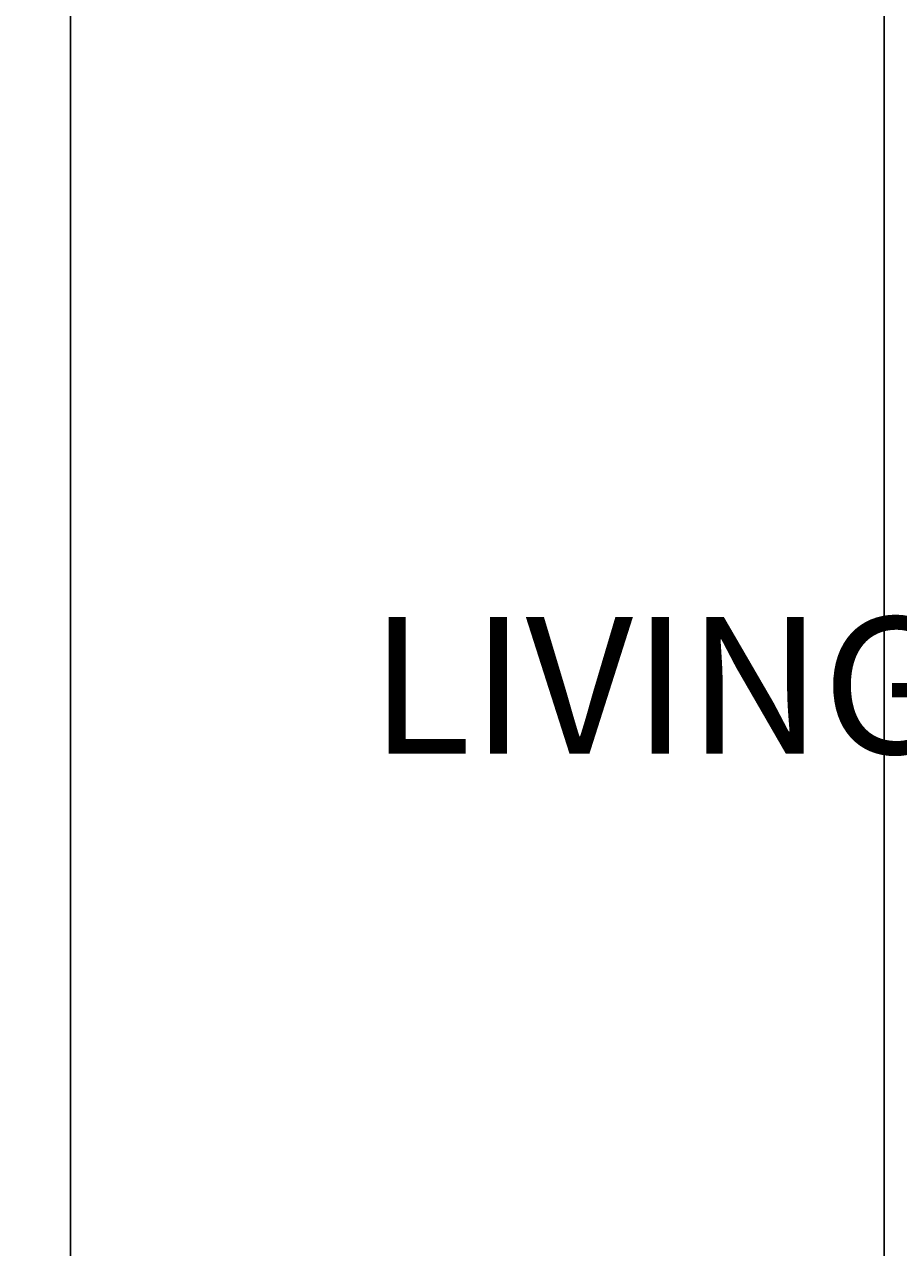
# Model space of a CAD drawing. Units: inches. Extents: x 857 to 1111, y 424 to 822.
# Tile 4 of 9: x 983 to 1031, y 600 to 668. Entities that reach past the tile are written whole.
import ezdxf

# ---------------------------------------------------------------- set-up
doc = ezdxf.new("R2010")
doc.units = ezdxf.units.IN
doc.layers.add('A-ANNO-DIMS', color=2, linetype='Continuous', lineweight=18)
doc.layers.add('A-AREA-IDEN', color=7, linetype='Continuous', lineweight=25)
doc.styles.get("Standard").update_dxf_attribs({"font": 'arial.ttf'})
doc.dimstyles.get("Standard").update_dxf_attribs({"dimtxt": 0.18, "dimasz": 0.18, "dimexe": 0.18, "dimexo": 0.0625, "dimgap": 0.09, "dimtad": 0, "dimtih": 1, "dimtoh": 1, "dimdec": 4, "dimzin": 0, "dimdsep": 46, "dimtxsty": 'Standard', "dimcen": 0.09, "dimadec": 0, "dimazin": 0, "dimtfac": 1, "dimtdec": 4, "dimtofl": 0, "dimtmove": 0, "dimatfit": 3, "dimfxl": 1, "dimtolj": 1, "dimtzin": 0, "dimarcsym": 0})

# ---------------------------------------------------------------- blocks, each defined once
blk = doc.blocks.new('*D48')
at = {"layer": 'A-ANNO-DIMS', "color": 0, "lineweight": -2, "transparency": 16777216}
for p, q in [((885.137, 582.419), (885.137, 822.087)), ((885.317, 821.907), (935.001, 821.907)), ((985.457, 821.907), (935.773, 821.907)), ((985.637, 582.419), (985.637, 822.087))]:
    blk.add_line(p, q, dxfattribs=at)
at = {"layer": 'A-ANNO-DIMS', "color": 0, "transparency": 16777216}
for points in [[(885.317, 821.937), (885.317, 821.877), (885.137, 821.907)], [(985.457, 821.937), (985.457, 821.877), (985.637, 821.907)]]:
    blk.add_solid(points, dxfattribs=at)
at = {"layer": 'Defpoints', "color": 0, "transparency": 16777216}
for p in [(985.637, 821.907), (885.137, 582.357), (985.637, 582.357)]:
    blk.add_point(p, dxfattribs=at)
at = {"layer": 'A-ANNO-DIMS', "color": 0, "transparency": 16777216, "insert": (935.387, 821.907), "char_height": 0.18, "attachment_point": 5}
blk.add_mtext('\\A1;100.5', dxfattribs=at)
blk = doc.blocks.new('*D49')
at = {"layer": 'A-ANNO-DIMS', "color": 0, "lineweight": -2, "transparency": 16777216}
for p, q in [((985.637, 451.919), (985.637, 822.087)), ((985.817, 821.907), (1007.914, 821.907)), ((1030.457, 821.907), (1008.36, 821.907)), ((1030.637, 451.919), (1030.637, 822.087))]:
    blk.add_line(p, q, dxfattribs=at)
at = {"layer": 'A-ANNO-DIMS', "color": 0, "transparency": 16777216}
for points in [[(985.817, 821.937), (985.817, 821.877), (985.637, 821.907)], [(1030.457, 821.937), (1030.457, 821.877), (1030.637, 821.907)]]:
    blk.add_solid(points, dxfattribs=at)
at = {"layer": 'Defpoints', "color": 0, "transparency": 16777216}
for p in [(1030.637, 821.907), (985.637, 451.857), (1030.637, 451.857)]:
    blk.add_point(p, dxfattribs=at)
at = {"layer": 'A-ANNO-DIMS', "color": 0, "transparency": 16777216, "insert": (1008.137, 821.907), "char_height": 0.18, "attachment_point": 5}
blk.add_mtext('\\A1;45', dxfattribs=at)
blk = doc.blocks.new('*D56')
at = {"layer": 'A-ANNO-DIMS', "color": 0, "lineweight": -2, "transparency": 16777216}
for p, q in [((924.77, 717.294), (924.77, 423.627)), ((1053.972, 717.294), (1053.972, 423.627)), ((924.95, 423.807), (988.986, 423.807)), ((1053.792, 423.807), (989.755, 423.807))]:
    blk.add_line(p, q, dxfattribs=at)
at = {"layer": 'A-ANNO-DIMS', "color": 0, "transparency": 16777216}
for points in [[(924.95, 423.837), (924.95, 423.777), (924.77, 423.807)], [(1053.792, 423.837), (1053.792, 423.777), (1053.972, 423.807)]]:
    blk.add_solid(points, dxfattribs=at)
at = {"layer": 'Defpoints', "color": 0, "transparency": 16777216}
for p in [(924.77, 717.357), (1053.972, 717.357), (1053.972, 423.807)]:
    blk.add_point(p, dxfattribs=at)
at = {"layer": 'A-ANNO-DIMS', "color": 0, "transparency": 16777216, "insert": (989.371, 423.807), "char_height": 0.18, "attachment_point": 5}
blk.add_mtext('\\A1;129.2', dxfattribs=at)

msp = doc.modelspace()

# ---------------------------------------------------------------- texts
at = {"layer": 'A-AREA-IDEN'}
msp.add_text('LIVING / DINING ', height=7.55928, dxfattribs=at).set_placement((1002.1837, 627.4375))

# ---------------------------------------------------------------- dimensions: what is measured, and where the dimension line sits
at = {"layer": 'A-ANNO-DIMS'}
for base, p1, p2, override, picture, middle in [((985.6369, 821.9067), (885.1369, 582.3567), (985.6369, 582.3567), {"dimdec": 1, "dimlfac": 1, "dimrnd": 0, "dimzin": 0, "dimdsep": 46, "dimlunit": 2}, '*D48', (935.3869, 821.9067)), ((1030.6369, 821.9067), (985.6369, 451.8567), (1030.6369, 451.8567), {"dimdec": 0, "dimlfac": 1, "dimrnd": 0, "dimzin": 0, "dimdsep": 46, "dimlunit": 2}, '*D49', (1008.1369, 821.9067)), ((1053.9717, 423.8067), (924.7696, 717.3567), (1053.9717, 717.3567), {"dimdec": 1, "dimlfac": 1, "dimrnd": 0, "dimzin": 0, "dimdsep": 46, "dimlunit": 2}, '*D56', (989.3707, 423.8067))]:
    dim = msp.add_linear_dim(base=base, p1=p1, p2=p2, dimstyle='Standard', override=override, dxfattribs=at)
    dim.commit()
    dim.dimension.update_dxf_attribs({"geometry": picture, "text_midpoint": middle})

doc.saveas('drawing.dxf')
